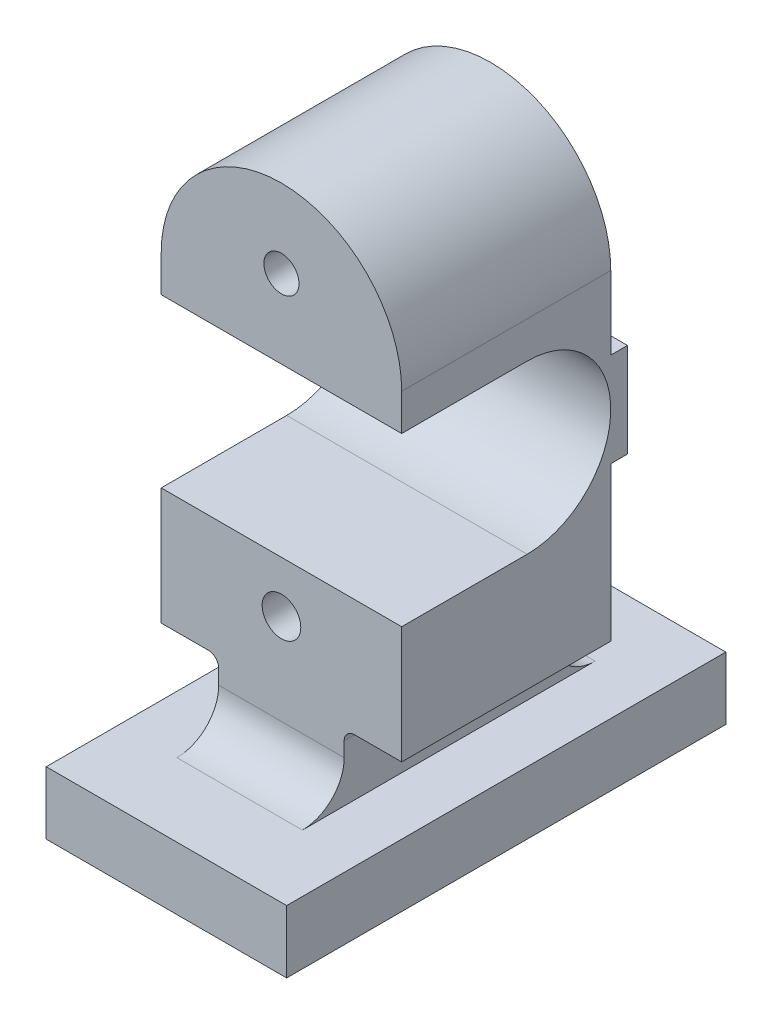
ISO-10303-21;
HEADER;
FILE_DESCRIPTION(('STEP AP214'),'2;1');
FILE_NAME('part.step','',(''),(''),'','','');
FILE_SCHEMA(('AUTOMOTIVE_DESIGN { 1 0 10303 214 1 1 1 1 }'));
ENDSEC;
DATA;
#1=APPLICATION_CONTEXT('core data for automotive mechanical design processes');
#2=APPLICATION_PROTOCOL_DEFINITION('international standard','automotive_design',2000,#1);
#3=PRODUCT_CONTEXT('',#1,'mechanical');
#4=PRODUCT('Part','Part','',(#3));
#5=PRODUCT_RELATED_PRODUCT_CATEGORY('part','',(#4));
#6=PRODUCT_DEFINITION_FORMATION('','',#4);
#7=PRODUCT_DEFINITION_CONTEXT('part definition',#1,'design');
#8=PRODUCT_DEFINITION('design','',#6,#7);
#9=PRODUCT_DEFINITION_SHAPE('','',#8);
#10=(LENGTH_UNIT() NAMED_UNIT(*) SI_UNIT(.MILLI.,.METRE.));
#11=(NAMED_UNIT(*) PLANE_ANGLE_UNIT() SI_UNIT($,.RADIAN.));
#12=(NAMED_UNIT(*) SI_UNIT($,.STERADIAN.) SOLID_ANGLE_UNIT());
#13=UNCERTAINTY_MEASURE_WITH_UNIT(LENGTH_MEASURE(1.E-05),#10,'distance_accuracy_value','');
#14=(GEOMETRIC_REPRESENTATION_CONTEXT(3) GLOBAL_UNCERTAINTY_ASSIGNED_CONTEXT((#13)) GLOBAL_UNIT_ASSIGNED_CONTEXT((#10,
#11,#12)) REPRESENTATION_CONTEXT('',''));
#15=CARTESIAN_POINT('',(0.,0.,0.));
#16=DIRECTION('',(0.,0.,1.));
#17=DIRECTION('',(1.,0.,0.));
#18=AXIS2_PLACEMENT_3D('',#15,#16,#17);
#19=CARTESIAN_POINT('',(35.0000000000001,42.,50.));
#20=DIRECTION('',(0.,0.,-1.));
#21=DIRECTION('',(-1.,0.,0.));
#22=AXIS2_PLACEMENT_3D('',#19,#20,#21);
#23=PLANE('',#22);
#24=CARTESIAN_POINT('',(0.,78.5,50.));
#25=DIRECTION('',(0.,0.,1.));
#26=DIRECTION('',(1.,0.,0.));
#27=AXIS2_PLACEMENT_3D('',#24,#25,#26);
#28=CIRCLE('',#27,9.24443485272175);
#29=CARTESIAN_POINT('',(9.24443485272181,78.5,50.));
#30=VERTEX_POINT('',#29);
#31=EDGE_CURVE('E348',#30,#30,#28,.T.);
#32=ORIENTED_EDGE('',*,*,#31,.F.);
#33=EDGE_LOOP('',(#32));
#34=FACE_BOUND('',#33,.T.);
#35=DIRECTION('',(0.,-1.,0.));
#36=VECTOR('',#35,1.);
#37=CARTESIAN_POINT('',(-29.9999999999999,42.,50.));
#38=LINE('',#37,#36);
#39=CARTESIAN_POINT('',(-29.9999999999999,42.,50.));
#40=VERTEX_POINT('',#39);
#41=CARTESIAN_POINT('',(-29.9999999999999,35.,50.));
#42=VERTEX_POINT('',#41);
#43=EDGE_CURVE('E361',#40,#42,#38,.T.);
#44=ORIENTED_EDGE('',*,*,#43,.T.);
#45=DIRECTION('',(1.,0.,0.));
#46=VECTOR('',#45,1.);
#47=CARTESIAN_POINT('',(35.0000000000001,35.,50.));
#48=LINE('',#47,#46);
#49=CARTESIAN_POINT('',(30.0000000000001,35.,50.));
#50=VERTEX_POINT('',#49);
#51=EDGE_CURVE('E393',#42,#50,#48,.T.);
#52=ORIENTED_EDGE('',*,*,#51,.T.);
#53=DIRECTION('',(0.,1.,0.));
#54=VECTOR('',#53,1.);
#55=CARTESIAN_POINT('',(30.0000000000001,42.,50.));
#56=LINE('',#55,#54);
#57=CARTESIAN_POINT('',(30.0000000000001,42.,50.));
#58=VERTEX_POINT('',#57);
#59=EDGE_CURVE('E363',#50,#58,#56,.T.);
#60=ORIENTED_EDGE('',*,*,#59,.T.);
#61=CARTESIAN_POINT('',(35.0000000000001,42.,50.));
#62=DIRECTION('',(0.,0.,-1.));
#63=DIRECTION('',(-1.,0.,0.));
#64=AXIS2_PLACEMENT_3D('',#61,#62,#63);
#65=CIRCLE('',#64,5.);
#66=CARTESIAN_POINT('',(35.0000000000001,47.,50.));
#67=VERTEX_POINT('',#66);
#68=EDGE_CURVE('E360',#58,#67,#65,.T.);
#69=ORIENTED_EDGE('',*,*,#68,.T.);
#70=DIRECTION('',(1.,0.,0.));
#71=VECTOR('',#70,1.);
#72=CARTESIAN_POINT('',(57.5,47.,50.));
#73=LINE('',#72,#71);
#74=CARTESIAN_POINT('',(57.5,47.,50.));
#75=VERTEX_POINT('',#74);
#76=EDGE_CURVE('E358',#67,#75,#73,.T.);
#77=ORIENTED_EDGE('',*,*,#76,.T.);
#78=DIRECTION('',(0.,1.,0.));
#79=VECTOR('',#78,1.);
#80=CARTESIAN_POINT('',(57.5,47.,50.));
#81=LINE('',#80,#79);
#82=CARTESIAN_POINT('',(57.5,103.,50.));
#83=VERTEX_POINT('',#82);
#84=EDGE_CURVE('E356',#75,#83,#81,.T.);
#85=ORIENTED_EDGE('',*,*,#84,.T.);
#86=DIRECTION('',(1.,0.,0.));
#87=VECTOR('',#86,1.);
#88=CARTESIAN_POINT('',(-75.,103.,50.));
#89=LINE('',#88,#87);
#90=CARTESIAN_POINT('',(-57.5,103.,50.));
#91=VERTEX_POINT('',#90);
#92=EDGE_CURVE('E373',#91,#83,#89,.T.);
#93=ORIENTED_EDGE('',*,*,#92,.F.);
#94=DIRECTION('',(0.,-1.,0.));
#95=VECTOR('',#94,1.);
#96=CARTESIAN_POINT('',(-57.5,47.,50.));
#97=LINE('',#96,#95);
#98=CARTESIAN_POINT('',(-57.5,47.,50.));
#99=VERTEX_POINT('',#98);
#100=EDGE_CURVE('E282',#91,#99,#97,.T.);
#101=ORIENTED_EDGE('',*,*,#100,.T.);
#102=DIRECTION('',(1.,0.,0.));
#103=VECTOR('',#102,1.);
#104=CARTESIAN_POINT('',(-34.9999999999999,47.,50.));
#105=LINE('',#104,#103);
#106=CARTESIAN_POINT('',(-34.9999999999999,47.,50.));
#107=VERTEX_POINT('',#106);
#108=EDGE_CURVE('E370',#99,#107,#105,.T.);
#109=ORIENTED_EDGE('',*,*,#108,.T.);
#110=CARTESIAN_POINT('',(-34.9999999999999,42.,50.));
#111=DIRECTION('',(0.,0.,-1.));
#112=DIRECTION('',(1.,0.,0.));
#113=AXIS2_PLACEMENT_3D('',#110,#111,#112);
#114=CIRCLE('',#113,5.);
#115=EDGE_CURVE('E362',#107,#40,#114,.T.);
#116=ORIENTED_EDGE('',*,*,#115,.T.);
#117=EDGE_LOOP('',(#44,#52,#60,#69,#77,#85,#93,#101,#109,#116));
#118=FACE_BOUND('',#117,.T.);
#119=ADVANCED_FACE('F41',(#34,#118),#23,.F.);
#120=CARTESIAN_POINT('',(35.0000000000001,42.,-50.));
#121=DIRECTION('',(0.,0.,-1.));
#122=DIRECTION('',(-1.,0.,0.));
#123=AXIS2_PLACEMENT_3D('',#120,#121,#122);
#124=PLANE('',#123);
#125=DIRECTION('',(0.,1.,0.));
#126=VECTOR('',#125,1.);
#127=CARTESIAN_POINT('',(30.0000000000001,42.,-50.));
#128=LINE('',#127,#126);
#129=CARTESIAN_POINT('',(30.0000000000001,35.,-50.));
#130=VERTEX_POINT('',#129);
#131=CARTESIAN_POINT('',(30.0000000000001,42.,-50.));
#132=VERTEX_POINT('',#131);
#133=EDGE_CURVE('E333',#130,#132,#128,.T.);
#134=ORIENTED_EDGE('',*,*,#133,.F.);
#135=DIRECTION('',(1.,0.,0.));
#136=VECTOR('',#135,1.);
#137=CARTESIAN_POINT('',(-29.9999999999999,35.,-50.));
#138=LINE('',#137,#136);
#139=CARTESIAN_POINT('',(-29.9999999999999,35.,-50.));
#140=VERTEX_POINT('',#139);
#141=EDGE_CURVE('E391',#130,#140,#138,.F.);
#142=ORIENTED_EDGE('',*,*,#141,.T.);
#143=DIRECTION('',(0.,-1.,0.));
#144=VECTOR('',#143,1.);
#145=CARTESIAN_POINT('',(-29.9999999999999,42.,-50.));
#146=LINE('',#145,#144);
#147=CARTESIAN_POINT('',(-29.9999999999999,42.,-50.));
#148=VERTEX_POINT('',#147);
#149=EDGE_CURVE('E327',#148,#140,#146,.T.);
#150=ORIENTED_EDGE('',*,*,#149,.F.);
#151=CARTESIAN_POINT('',(-34.9999999999999,42.,-50.));
#152=DIRECTION('',(0.,0.,-1.));
#153=DIRECTION('',(1.,0.,0.));
#154=AXIS2_PLACEMENT_3D('',#151,#152,#153);
#155=CIRCLE('',#154,5.);
#156=CARTESIAN_POINT('',(-34.9999999999999,47.,-50.));
#157=VERTEX_POINT('',#156);
#158=EDGE_CURVE('E321',#157,#148,#155,.T.);
#159=ORIENTED_EDGE('',*,*,#158,.F.);
#160=DIRECTION('',(1.,0.,0.));
#161=VECTOR('',#160,1.);
#162=CARTESIAN_POINT('',(-34.9999999999999,47.,-50.));
#163=LINE('',#162,#161);
#164=CARTESIAN_POINT('',(-57.5,47.,-50.));
#165=VERTEX_POINT('',#164);
#166=EDGE_CURVE('E323',#165,#157,#163,.T.);
#167=ORIENTED_EDGE('',*,*,#166,.F.);
#168=DIRECTION('',(0.,-1.,0.));
#169=VECTOR('',#168,1.);
#170=CARTESIAN_POINT('',(-57.5,47.,-50.));
#171=LINE('',#170,#169);
#172=CARTESIAN_POINT('',(-57.5,120.5,-50.));
#173=VERTEX_POINT('',#172);
#174=EDGE_CURVE('E211',#173,#165,#171,.T.);
#175=ORIENTED_EDGE('',*,*,#174,.F.);
#176=DIRECTION('',(-1.,0.,0.));
#177=VECTOR('',#176,1.);
#178=CARTESIAN_POINT('',(57.5,120.5,-50.));
#179=LINE('',#178,#177);
#180=CARTESIAN_POINT('',(57.5,120.5,-50.));
#181=VERTEX_POINT('',#180);
#182=EDGE_CURVE('E273',#181,#173,#179,.T.);
#183=ORIENTED_EDGE('',*,*,#182,.F.);
#184=DIRECTION('',(0.,1.,0.));
#185=VECTOR('',#184,1.);
#186=CARTESIAN_POINT('',(57.5,47.,-50.));
#187=LINE('',#186,#185);
#188=CARTESIAN_POINT('',(57.5,47.,-50.));
#189=VERTEX_POINT('',#188);
#190=EDGE_CURVE('E343',#189,#181,#187,.T.);
#191=ORIENTED_EDGE('',*,*,#190,.F.);
#192=DIRECTION('',(1.,0.,0.));
#193=VECTOR('',#192,1.);
#194=CARTESIAN_POINT('',(57.5,47.,-50.));
#195=LINE('',#194,#193);
#196=CARTESIAN_POINT('',(35.0000000000001,47.,-50.));
#197=VERTEX_POINT('',#196);
#198=EDGE_CURVE('E342',#197,#189,#195,.T.);
#199=ORIENTED_EDGE('',*,*,#198,.F.);
#200=CARTESIAN_POINT('',(35.0000000000001,42.,-50.));
#201=DIRECTION('',(0.,0.,-1.));
#202=DIRECTION('',(-1.,0.,0.));
#203=AXIS2_PLACEMENT_3D('',#200,#201,#202);
#204=CIRCLE('',#203,5.);
#205=EDGE_CURVE('E340',#132,#197,#204,.T.);
#206=ORIENTED_EDGE('',*,*,#205,.F.);
#207=EDGE_LOOP('',(#134,#142,#150,#159,#167,#175,#183,#191,#199,#206));
#208=FACE_BOUND('',#207,.T.);
#209=CARTESIAN_POINT('',(0.,78.5,-50.));
#210=DIRECTION('',(0.,0.,1.));
#211=DIRECTION('',(1.,0.,0.));
#212=AXIS2_PLACEMENT_3D('',#209,#210,#211);
#213=CIRCLE('',#212,9.24443485272175);
#214=CARTESIAN_POINT('',(9.24443485272181,78.5,-50.));
#215=VERTEX_POINT('',#214);
#216=EDGE_CURVE('E318',#215,#215,#213,.T.);
#217=ORIENTED_EDGE('',*,*,#216,.T.);
#218=EDGE_LOOP('',(#217));
#219=FACE_BOUND('',#218,.T.);
#220=ADVANCED_FACE('F412',(#208,#219),#124,.T.);
#221=CARTESIAN_POINT('',(0.,15.,0.));
#222=DIRECTION('',(0.,1.,0.));
#223=DIRECTION('',(0.,0.,1.));
#224=AXIS2_PLACEMENT_3D('',#221,#222,#223);
#225=PLANE('',#224);
#226=DIRECTION('',(0.,0.,-1.));
#227=VECTOR('',#226,1.);
#228=CARTESIAN_POINT('',(57.5,15.,-105.));
#229=LINE('',#228,#227);
#230=CARTESIAN_POINT('',(57.5,15.,105.));
#231=VERTEX_POINT('',#230);
#232=CARTESIAN_POINT('',(57.5,15.,-105.));
#233=VERTEX_POINT('',#232);
#234=EDGE_CURVE('E320',#231,#233,#229,.T.);
#235=ORIENTED_EDGE('',*,*,#234,.T.);
#236=DIRECTION('',(-1.,0.,0.));
#237=VECTOR('',#236,1.);
#238=CARTESIAN_POINT('',(-57.5,15.,-105.));
#239=LINE('',#238,#237);
#240=CARTESIAN_POINT('',(-57.5,15.,-105.));
#241=VERTEX_POINT('',#240);
#242=EDGE_CURVE('E314',#233,#241,#239,.T.);
#243=ORIENTED_EDGE('',*,*,#242,.T.);
#244=DIRECTION('',(0.,0.,1.));
#245=VECTOR('',#244,1.);
#246=CARTESIAN_POINT('',(-57.5,15.,-105.));
#247=LINE('',#246,#245);
#248=CARTESIAN_POINT('',(-57.5,15.,105.));
#249=VERTEX_POINT('',#248);
#250=EDGE_CURVE('E312',#241,#249,#247,.T.);
#251=ORIENTED_EDGE('',*,*,#250,.T.);
#252=DIRECTION('',(1.,0.,0.));
#253=VECTOR('',#252,1.);
#254=CARTESIAN_POINT('',(-57.5,15.,105.));
#255=LINE('',#254,#253);
#256=EDGE_CURVE('E311',#249,#231,#255,.T.);
#257=ORIENTED_EDGE('',*,*,#256,.T.);
#258=EDGE_LOOP('',(#235,#243,#251,#257));
#259=FACE_BOUND('',#258,.T.);
#260=DIRECTION('',(1.,0.,0.));
#261=VECTOR('',#260,1.);
#262=CARTESIAN_POINT('',(30.0000000000001,15.,-70.));
#263=LINE('',#262,#261);
#264=CARTESIAN_POINT('',(-29.9999999999999,15.,-70.));
#265=VERTEX_POINT('',#264);
#266=CARTESIAN_POINT('',(30.0000000000001,15.,-70.));
#267=VERTEX_POINT('',#266);
#268=EDGE_CURVE('E389',#265,#267,#263,.T.);
#269=ORIENTED_EDGE('',*,*,#268,.T.);
#270=DIRECTION('',(0.,0.,-1.));
#271=VECTOR('',#270,1.);
#272=CARTESIAN_POINT('',(30.0000000000001,15.,50.));
#273=LINE('',#272,#271);
#274=CARTESIAN_POINT('',(30.0000000000001,15.,70.));
#275=VERTEX_POINT('',#274);
#276=EDGE_CURVE('E331',#275,#267,#273,.T.);
#277=ORIENTED_EDGE('',*,*,#276,.F.);
#278=DIRECTION('',(1.,0.,0.));
#279=VECTOR('',#278,1.);
#280=CARTESIAN_POINT('',(0.,15.,70.));
#281=LINE('',#280,#279);
#282=CARTESIAN_POINT('',(-29.9999999999999,15.,70.));
#283=VERTEX_POINT('',#282);
#284=EDGE_CURVE('E377',#275,#283,#281,.F.);
#285=ORIENTED_EDGE('',*,*,#284,.T.);
#286=DIRECTION('',(0.,0.,-1.));
#287=VECTOR('',#286,1.);
#288=CARTESIAN_POINT('',(-29.9999999999999,15.,50.));
#289=LINE('',#288,#287);
#290=EDGE_CURVE('E309',#283,#265,#289,.T.);
#291=ORIENTED_EDGE('',*,*,#290,.T.);
#292=EDGE_LOOP('',(#269,#277,#285,#291));
#293=FACE_BOUND('',#292,.T.);
#294=ADVANCED_FACE('F403',(#259,#293),#225,.T.);
#295=CARTESIAN_POINT('',(57.5,15.,-105.));
#296=DIRECTION('',(-1.,0.,0.));
#297=DIRECTION('',(0.,0.,1.));
#298=AXIS2_PLACEMENT_3D('',#295,#296,#297);
#299=PLANE('',#298);
#300=DIRECTION('',(0.,0.,-1.));
#301=VECTOR('',#300,1.);
#302=CARTESIAN_POINT('',(57.5,-15.,-105.));
#303=LINE('',#302,#301);
#304=CARTESIAN_POINT('',(57.5,-15.,105.));
#305=VERTEX_POINT('',#304);
#306=CARTESIAN_POINT('',(57.5,-15.,-105.));
#307=VERTEX_POINT('',#306);
#308=EDGE_CURVE('E302',#305,#307,#303,.T.);
#309=ORIENTED_EDGE('',*,*,#308,.T.);
#310=DIRECTION('',(0.,-1.,0.));
#311=VECTOR('',#310,1.);
#312=CARTESIAN_POINT('',(57.5,15.,-105.));
#313=LINE('',#312,#311);
#314=EDGE_CURVE('E289',#233,#307,#313,.T.);
#315=ORIENTED_EDGE('',*,*,#314,.F.);
#316=ORIENTED_EDGE('',*,*,#234,.F.);
#317=DIRECTION('',(0.,-1.,0.));
#318=VECTOR('',#317,1.);
#319=CARTESIAN_POINT('',(57.5,15.,105.));
#320=LINE('',#319,#318);
#321=EDGE_CURVE('E301',#231,#305,#320,.T.);
#322=ORIENTED_EDGE('',*,*,#321,.T.);
#323=EDGE_LOOP('',(#309,#315,#316,#322));
#324=FACE_BOUND('',#323,.T.);
#325=ADVANCED_FACE('F511',(#324),#299,.F.);
#326=CARTESIAN_POINT('',(-57.5,15.,-105.));
#327=DIRECTION('',(0.,0.,1.));
#328=DIRECTION('',(1.,0.,0.));
#329=AXIS2_PLACEMENT_3D('',#326,#327,#328);
#330=PLANE('',#329);
#331=DIRECTION('',(-1.,0.,0.));
#332=VECTOR('',#331,1.);
#333=CARTESIAN_POINT('',(-57.5,-15.,-105.));
#334=LINE('',#333,#332);
#335=CARTESIAN_POINT('',(-57.5,-15.,-105.));
#336=VERTEX_POINT('',#335);
#337=EDGE_CURVE('E291',#307,#336,#334,.T.);
#338=ORIENTED_EDGE('',*,*,#337,.T.);
#339=DIRECTION('',(0.,-1.,0.));
#340=VECTOR('',#339,1.);
#341=CARTESIAN_POINT('',(-57.5,15.,-105.));
#342=LINE('',#341,#340);
#343=EDGE_CURVE('E295',#241,#336,#342,.T.);
#344=ORIENTED_EDGE('',*,*,#343,.F.);
#345=ORIENTED_EDGE('',*,*,#242,.F.);
#346=ORIENTED_EDGE('',*,*,#314,.T.);
#347=EDGE_LOOP('',(#338,#344,#345,#346));
#348=FACE_BOUND('',#347,.T.);
#349=ADVANCED_FACE('F520',(#348),#330,.F.);
#350=CARTESIAN_POINT('',(-57.5,15.,-105.));
#351=DIRECTION('',(1.,0.,0.));
#352=DIRECTION('',(0.,0.,-1.));
#353=AXIS2_PLACEMENT_3D('',#350,#351,#352);
#354=PLANE('',#353);
#355=DIRECTION('',(0.,0.,1.));
#356=VECTOR('',#355,1.);
#357=CARTESIAN_POINT('',(-57.5,-15.,-105.));
#358=LINE('',#357,#356);
#359=CARTESIAN_POINT('',(-57.5,-15.,105.));
#360=VERTEX_POINT('',#359);
#361=EDGE_CURVE('E292',#336,#360,#358,.T.);
#362=ORIENTED_EDGE('',*,*,#361,.T.);
#363=DIRECTION('',(0.,-1.,0.));
#364=VECTOR('',#363,1.);
#365=CARTESIAN_POINT('',(-57.5,15.,105.));
#366=LINE('',#365,#364);
#367=EDGE_CURVE('E296',#249,#360,#366,.T.);
#368=ORIENTED_EDGE('',*,*,#367,.F.);
#369=ORIENTED_EDGE('',*,*,#250,.F.);
#370=ORIENTED_EDGE('',*,*,#343,.T.);
#371=EDGE_LOOP('',(#362,#368,#369,#370));
#372=FACE_BOUND('',#371,.T.);
#373=ADVANCED_FACE('F521',(#372),#354,.F.);
#374=CARTESIAN_POINT('',(-57.5,15.,105.));
#375=DIRECTION('',(0.,0.,-1.));
#376=DIRECTION('',(-1.,0.,0.));
#377=AXIS2_PLACEMENT_3D('',#374,#375,#376);
#378=PLANE('',#377);
#379=DIRECTION('',(1.,0.,0.));
#380=VECTOR('',#379,1.);
#381=CARTESIAN_POINT('',(-57.5,-15.,105.));
#382=LINE('',#381,#380);
#383=EDGE_CURVE('E300',#360,#305,#382,.T.);
#384=ORIENTED_EDGE('',*,*,#383,.T.);
#385=ORIENTED_EDGE('',*,*,#321,.F.);
#386=ORIENTED_EDGE('',*,*,#256,.F.);
#387=ORIENTED_EDGE('',*,*,#367,.T.);
#388=EDGE_LOOP('',(#384,#385,#386,#387));
#389=FACE_BOUND('',#388,.T.);
#390=ADVANCED_FACE('F524',(#389),#378,.F.);
#391=CARTESIAN_POINT('',(0.,-15.,0.));
#392=DIRECTION('',(0.,1.,0.));
#393=DIRECTION('',(0.,0.,1.));
#394=AXIS2_PLACEMENT_3D('',#391,#392,#393);
#395=PLANE('',#394);
#396=ORIENTED_EDGE('',*,*,#308,.F.);
#397=ORIENTED_EDGE('',*,*,#383,.F.);
#398=ORIENTED_EDGE('',*,*,#361,.F.);
#399=ORIENTED_EDGE('',*,*,#337,.F.);
#400=EDGE_LOOP('',(#396,#397,#398,#399));
#401=FACE_BOUND('',#400,.T.);
#402=ADVANCED_FACE('F529',(#401),#395,.F.);
#403=CARTESIAN_POINT('',(-57.5,47.,50.));
#404=DIRECTION('',(1.,0.,0.));
#405=DIRECTION('',(0.,1.,0.));
#406=AXIS2_PLACEMENT_3D('',#403,#404,#405);
#407=PLANE('',#406);
#408=DIRECTION('',(0.,0.,-1.));
#409=VECTOR('',#408,1.);
#410=CARTESIAN_POINT('',(-57.5,103.,50.));
#411=LINE('',#410,#409);
#412=CARTESIAN_POINT('',(-57.5,103.,-9.99999999999999));
#413=VERTEX_POINT('',#412);
#414=EDGE_CURVE('E209',#91,#413,#411,.T.);
#415=ORIENTED_EDGE('',*,*,#414,.T.);
#416=CARTESIAN_POINT('',(-57.5,143.,-10.));
#417=DIRECTION('',(1.,0.,0.));
#418=DIRECTION('',(0.,1.,0.));
#419=AXIS2_PLACEMENT_3D('',#416,#417,#418);
#420=CIRCLE('',#419,40.);
#421=CARTESIAN_POINT('',(-57.5,183.,-9.99999999999999));
#422=VERTEX_POINT('',#421);
#423=EDGE_CURVE('E205',#413,#422,#420,.T.);
#424=ORIENTED_EDGE('',*,*,#423,.T.);
#425=DIRECTION('',(0.,0.,1.));
#426=VECTOR('',#425,1.);
#427=CARTESIAN_POINT('',(-57.5,183.,50.));
#428=LINE('',#427,#426);
#429=CARTESIAN_POINT('',(-57.5,183.,50.));
#430=VERTEX_POINT('',#429);
#431=EDGE_CURVE('E207',#422,#430,#428,.T.);
#432=ORIENTED_EDGE('',*,*,#431,.T.);
#433=DIRECTION('',(0.,-1.,0.));
#434=VECTOR('',#433,1.);
#435=CARTESIAN_POINT('',(-57.5,47.,50.));
#436=LINE('',#435,#434);
#437=CARTESIAN_POINT('',(-57.5,200.5,50.));
#438=VERTEX_POINT('',#437);
#439=EDGE_CURVE('E240',#438,#430,#436,.T.);
#440=ORIENTED_EDGE('',*,*,#439,.F.);
#441=DIRECTION('',(0.,0.,-1.));
#442=VECTOR('',#441,1.);
#443=CARTESIAN_POINT('',(-57.5,200.5,50.));
#444=LINE('',#443,#442);
#445=CARTESIAN_POINT('',(-57.5,200.5,-50.));
#446=VERTEX_POINT('',#445);
#447=EDGE_CURVE('E245',#438,#446,#444,.T.);
#448=ORIENTED_EDGE('',*,*,#447,.T.);
#449=DIRECTION('',(0.,-1.,0.));
#450=VECTOR('',#449,1.);
#451=CARTESIAN_POINT('',(-57.5,47.,-50.));
#452=LINE('',#451,#450);
#453=CARTESIAN_POINT('',(-57.5,165.5,-50.));
#454=VERTEX_POINT('',#453);
#455=EDGE_CURVE('E234',#446,#454,#452,.T.);
#456=ORIENTED_EDGE('',*,*,#455,.T.);
#457=DIRECTION('',(0.,0.,1.));
#458=VECTOR('',#457,1.);
#459=CARTESIAN_POINT('',(-57.5,165.5,-50.));
#460=LINE('',#459,#458);
#461=CARTESIAN_POINT('',(-57.5,165.5,-58.));
#462=VERTEX_POINT('',#461);
#463=EDGE_CURVE('E266',#462,#454,#460,.T.);
#464=ORIENTED_EDGE('',*,*,#463,.F.);
#465=DIRECTION('',(0.,1.,0.));
#466=VECTOR('',#465,1.);
#467=CARTESIAN_POINT('',(-57.5,120.5,-58.));
#468=LINE('',#467,#466);
#469=CARTESIAN_POINT('',(-57.5,120.5,-58.));
#470=VERTEX_POINT('',#469);
#471=EDGE_CURVE('E259',#470,#462,#468,.T.);
#472=ORIENTED_EDGE('',*,*,#471,.F.);
#473=DIRECTION('',(0.,0.,-1.));
#474=VECTOR('',#473,1.);
#475=CARTESIAN_POINT('',(-57.5,120.5,-50.));
#476=LINE('',#475,#474);
#477=EDGE_CURVE('E263',#173,#470,#476,.T.);
#478=ORIENTED_EDGE('',*,*,#477,.F.);
#479=ORIENTED_EDGE('',*,*,#174,.T.);
#480=DIRECTION('',(0.,0.,-1.));
#481=VECTOR('',#480,1.);
#482=CARTESIAN_POINT('',(-57.5,47.,50.));
#483=LINE('',#482,#481);
#484=EDGE_CURVE('E322',#99,#165,#483,.T.);
#485=ORIENTED_EDGE('',*,*,#484,.F.);
#486=ORIENTED_EDGE('',*,*,#100,.F.);
#487=EDGE_LOOP('',(#415,#424,#432,#440,#448,#456,#464,#472,#478,#479,#485,#486));
#488=FACE_BOUND('',#487,.T.);
#489=ADVANCED_FACE('F204',(#488),#407,.F.);
#490=CARTESIAN_POINT('',(-34.9999999999999,47.,50.));
#491=DIRECTION('',(0.,1.,0.));
#492=DIRECTION('',(-1.,0.,0.));
#493=AXIS2_PLACEMENT_3D('',#490,#491,#492);
#494=PLANE('',#493);
#495=ORIENTED_EDGE('',*,*,#166,.T.);
#496=DIRECTION('',(0.,0.,-1.));
#497=VECTOR('',#496,1.);
#498=CARTESIAN_POINT('',(-34.9999999999999,47.,50.));
#499=LINE('',#498,#497);
#500=EDGE_CURVE('E326',#107,#157,#499,.T.);
#501=ORIENTED_EDGE('',*,*,#500,.F.);
#502=ORIENTED_EDGE('',*,*,#108,.F.);
#503=ORIENTED_EDGE('',*,*,#484,.T.);
#504=EDGE_LOOP('',(#495,#501,#502,#503));
#505=FACE_BOUND('',#504,.T.);
#506=ADVANCED_FACE('F439',(#505),#494,.F.);
#507=CARTESIAN_POINT('',(-34.9999999999999,42.,50.));
#508=DIRECTION('',(0.,0.,-1.));
#509=DIRECTION('',(-1.,0.,0.));
#510=AXIS2_PLACEMENT_3D('',#507,#508,#509);
#511=CYLINDRICAL_SURFACE('',#510,5.);
#512=ORIENTED_EDGE('',*,*,#158,.T.);
#513=DIRECTION('',(0.,0.,-1.));
#514=VECTOR('',#513,1.);
#515=CARTESIAN_POINT('',(-29.9999999999999,42.,50.));
#516=LINE('',#515,#514);
#517=EDGE_CURVE('E329',#40,#148,#516,.T.);
#518=ORIENTED_EDGE('',*,*,#517,.F.);
#519=ORIENTED_EDGE('',*,*,#115,.F.);
#520=ORIENTED_EDGE('',*,*,#500,.T.);
#521=EDGE_LOOP('',(#512,#518,#519,#520));
#522=FACE_BOUND('',#521,.T.);
#523=ADVANCED_FACE('F436',(#522),#511,.F.);
#524=CARTESIAN_POINT('',(-29.9999999999999,42.,50.));
#525=DIRECTION('',(1.,0.,0.));
#526=DIRECTION('',(0.,1.,0.));
#527=AXIS2_PLACEMENT_3D('',#524,#525,#526);
#528=PLANE('',#527);
#529=ORIENTED_EDGE('',*,*,#149,.T.);
#530=CARTESIAN_POINT('',(-29.9999999999999,35.,-70.));
#531=DIRECTION('',(1.,0.,0.));
#532=DIRECTION('',(0.,1.,0.));
#533=AXIS2_PLACEMENT_3D('',#530,#531,#532);
#534=CIRCLE('',#533,20.);
#535=EDGE_CURVE('E400',#140,#265,#534,.T.);
#536=ORIENTED_EDGE('',*,*,#535,.T.);
#537=ORIENTED_EDGE('',*,*,#290,.F.);
#538=CARTESIAN_POINT('',(-29.9999999999999,35.,70.));
#539=DIRECTION('',(1.,0.,0.));
#540=DIRECTION('',(0.,1.,0.));
#541=AXIS2_PLACEMENT_3D('',#538,#539,#540);
#542=CIRCLE('',#541,20.);
#543=EDGE_CURVE('E11',#283,#42,#542,.T.);
#544=ORIENTED_EDGE('',*,*,#543,.T.);
#545=ORIENTED_EDGE('',*,*,#43,.F.);
#546=ORIENTED_EDGE('',*,*,#517,.T.);
#547=EDGE_LOOP('',(#529,#536,#537,#544,#545,#546));
#548=FACE_BOUND('',#547,.T.);
#549=ADVANCED_FACE('F435',(#548),#528,.F.);
#550=CARTESIAN_POINT('',(30.0000000000001,42.,50.));
#551=DIRECTION('',(-1.,0.,0.));
#552=DIRECTION('',(0.,0.,1.));
#553=AXIS2_PLACEMENT_3D('',#550,#551,#552);
#554=PLANE('',#553);
#555=ORIENTED_EDGE('',*,*,#276,.T.);
#556=CARTESIAN_POINT('',(30.0000000000001,35.,-70.));
#557=DIRECTION('',(-1.,0.,0.));
#558=DIRECTION('',(0.,0.,1.));
#559=AXIS2_PLACEMENT_3D('',#556,#557,#558);
#560=CIRCLE('',#559,20.);
#561=EDGE_CURVE('E394',#267,#130,#560,.T.);
#562=ORIENTED_EDGE('',*,*,#561,.T.);
#563=ORIENTED_EDGE('',*,*,#133,.T.);
#564=DIRECTION('',(0.,0.,-1.));
#565=VECTOR('',#564,1.);
#566=CARTESIAN_POINT('',(30.0000000000001,42.,50.));
#567=LINE('',#566,#565);
#568=EDGE_CURVE('E336',#58,#132,#567,.T.);
#569=ORIENTED_EDGE('',*,*,#568,.F.);
#570=ORIENTED_EDGE('',*,*,#59,.F.);
#571=CARTESIAN_POINT('',(30.0000000000001,35.,70.));
#572=DIRECTION('',(-1.,0.,0.));
#573=DIRECTION('',(0.,0.,1.));
#574=AXIS2_PLACEMENT_3D('',#571,#572,#573);
#575=CIRCLE('',#574,20.);
#576=EDGE_CURVE('E47',#50,#275,#575,.T.);
#577=ORIENTED_EDGE('',*,*,#576,.T.);
#578=EDGE_LOOP('',(#555,#562,#563,#569,#570,#577));
#579=FACE_BOUND('',#578,.T.);
#580=ADVANCED_FACE('F402',(#579),#554,.F.);
#581=CARTESIAN_POINT('',(35.0000000000001,42.,50.));
#582=DIRECTION('',(0.,0.,-1.));
#583=DIRECTION('',(-1.,0.,0.));
#584=AXIS2_PLACEMENT_3D('',#581,#582,#583);
#585=CYLINDRICAL_SURFACE('',#584,5.);
#586=ORIENTED_EDGE('',*,*,#205,.T.);
#587=DIRECTION('',(0.,0.,-1.));
#588=VECTOR('',#587,1.);
#589=CARTESIAN_POINT('',(35.0000000000001,47.,50.));
#590=LINE('',#589,#588);
#591=EDGE_CURVE('E345',#67,#197,#590,.T.);
#592=ORIENTED_EDGE('',*,*,#591,.F.);
#593=ORIENTED_EDGE('',*,*,#68,.F.);
#594=ORIENTED_EDGE('',*,*,#568,.T.);
#595=EDGE_LOOP('',(#586,#592,#593,#594));
#596=FACE_BOUND('',#595,.T.);
#597=ADVANCED_FACE('F423',(#596),#585,.F.);
#598=CARTESIAN_POINT('',(57.5,47.,50.));
#599=DIRECTION('',(0.,1.,0.));
#600=DIRECTION('',(-1.,0.,0.));
#601=AXIS2_PLACEMENT_3D('',#598,#599,#600);
#602=PLANE('',#601);
#603=ORIENTED_EDGE('',*,*,#198,.T.);
#604=DIRECTION('',(0.,0.,-1.));
#605=VECTOR('',#604,1.);
#606=CARTESIAN_POINT('',(57.5,47.,50.));
#607=LINE('',#606,#605);
#608=EDGE_CURVE('E288',#75,#189,#607,.T.);
#609=ORIENTED_EDGE('',*,*,#608,.F.);
#610=ORIENTED_EDGE('',*,*,#76,.F.);
#611=ORIENTED_EDGE('',*,*,#591,.T.);
#612=EDGE_LOOP('',(#603,#609,#610,#611));
#613=FACE_BOUND('',#612,.T.);
#614=ADVANCED_FACE('F424',(#613),#602,.F.);
#615=CARTESIAN_POINT('',(57.5,47.,50.));
#616=DIRECTION('',(-1.,0.,0.));
#617=DIRECTION('',(0.,-1.,0.));
#618=AXIS2_PLACEMENT_3D('',#615,#616,#617);
#619=PLANE('',#618);
#620=ORIENTED_EDGE('',*,*,#190,.T.);
#621=DIRECTION('',(0.,0.,-1.));
#622=VECTOR('',#621,1.);
#623=CARTESIAN_POINT('',(57.5,120.5,-50.));
#624=LINE('',#623,#622);
#625=CARTESIAN_POINT('',(57.5,120.5,-58.));
#626=VERTEX_POINT('',#625);
#627=EDGE_CURVE('E264',#181,#626,#624,.T.);
#628=ORIENTED_EDGE('',*,*,#627,.T.);
#629=DIRECTION('',(0.,1.,0.));
#630=VECTOR('',#629,1.);
#631=CARTESIAN_POINT('',(57.5,120.5,-58.));
#632=LINE('',#631,#630);
#633=CARTESIAN_POINT('',(57.5,165.5,-58.));
#634=VERTEX_POINT('',#633);
#635=EDGE_CURVE('E256',#626,#634,#632,.T.);
#636=ORIENTED_EDGE('',*,*,#635,.T.);
#637=DIRECTION('',(0.,0.,1.));
#638=VECTOR('',#637,1.);
#639=CARTESIAN_POINT('',(57.5,165.5,-50.));
#640=LINE('',#639,#638);
#641=CARTESIAN_POINT('',(57.5,165.5,-50.));
#642=VERTEX_POINT('',#641);
#643=EDGE_CURVE('E265',#634,#642,#640,.T.);
#644=ORIENTED_EDGE('',*,*,#643,.T.);
#645=DIRECTION('',(0.,1.,0.));
#646=VECTOR('',#645,1.);
#647=CARTESIAN_POINT('',(57.5,47.,-50.));
#648=LINE('',#647,#646);
#649=CARTESIAN_POINT('',(57.5,200.5,-50.));
#650=VERTEX_POINT('',#649);
#651=EDGE_CURVE('E239',#642,#650,#648,.T.);
#652=ORIENTED_EDGE('',*,*,#651,.T.);
#653=DIRECTION('',(0.,0.,-1.));
#654=VECTOR('',#653,1.);
#655=CARTESIAN_POINT('',(57.5,200.5,50.));
#656=LINE('',#655,#654);
#657=CARTESIAN_POINT('',(57.5,200.5,50.));
#658=VERTEX_POINT('',#657);
#659=EDGE_CURVE('E247',#650,#658,#656,.F.);
#660=ORIENTED_EDGE('',*,*,#659,.T.);
#661=DIRECTION('',(0.,1.,0.));
#662=VECTOR('',#661,1.);
#663=CARTESIAN_POINT('',(57.5,47.,50.));
#664=LINE('',#663,#662);
#665=CARTESIAN_POINT('',(57.5,183.,50.));
#666=VERTEX_POINT('',#665);
#667=EDGE_CURVE('E237',#666,#658,#664,.T.);
#668=ORIENTED_EDGE('',*,*,#667,.F.);
#669=DIRECTION('',(0.,0.,-1.));
#670=VECTOR('',#669,1.);
#671=CARTESIAN_POINT('',(57.5,183.,50.));
#672=LINE('',#671,#670);
#673=CARTESIAN_POINT('',(57.5,183.,-9.99999999999999));
#674=VERTEX_POINT('',#673);
#675=EDGE_CURVE('E257',#666,#674,#672,.T.);
#676=ORIENTED_EDGE('',*,*,#675,.T.);
#677=CARTESIAN_POINT('',(57.5,143.,-10.));
#678=DIRECTION('',(-1.,0.,0.));
#679=DIRECTION('',(0.,-1.,0.));
#680=AXIS2_PLACEMENT_3D('',#677,#678,#679);
#681=CIRCLE('',#680,40.);
#682=CARTESIAN_POINT('',(57.5,103.,-9.99999999999999));
#683=VERTEX_POINT('',#682);
#684=EDGE_CURVE('E227',#674,#683,#681,.T.);
#685=ORIENTED_EDGE('',*,*,#684,.T.);
#686=DIRECTION('',(0.,0.,1.));
#687=VECTOR('',#686,1.);
#688=CARTESIAN_POINT('',(57.5,103.,50.));
#689=LINE('',#688,#687);
#690=EDGE_CURVE('E284',#683,#83,#689,.T.);
#691=ORIENTED_EDGE('',*,*,#690,.T.);
#692=ORIENTED_EDGE('',*,*,#84,.F.);
#693=ORIENTED_EDGE('',*,*,#608,.T.);
#694=EDGE_LOOP('',(#620,#628,#636,#644,#652,#660,#668,#676,#685,#691,#692,#693));
#695=FACE_BOUND('',#694,.T.);
#696=ADVANCED_FACE('F448',(#695),#619,.F.);
#697=CARTESIAN_POINT('',(0.,78.5,50.));
#698=DIRECTION('',(0.,0.,-1.));
#699=DIRECTION('',(-1.,0.,0.));
#700=AXIS2_PLACEMENT_3D('',#697,#698,#699);
#701=CYLINDRICAL_SURFACE('',#700,9.24443485272175);
#702=ORIENTED_EDGE('',*,*,#31,.T.);
#703=EDGE_LOOP('',(#702));
#704=FACE_BOUND('',#703,.T.);
#705=ORIENTED_EDGE('',*,*,#216,.F.);
#706=EDGE_LOOP('',(#705));
#707=FACE_BOUND('',#706,.T.);
#708=ADVANCED_FACE('F453',(#704,#707),#701,.F.);
#709=CARTESIAN_POINT('',(-75.,103.,50.));
#710=DIRECTION('',(0.,-1.,0.));
#711=DIRECTION('',(0.,0.,-1.));
#712=AXIS2_PLACEMENT_3D('',#709,#710,#711);
#713=PLANE('',#712);
#714=ORIENTED_EDGE('',*,*,#92,.T.);
#715=ORIENTED_EDGE('',*,*,#690,.F.);
#716=DIRECTION('',(1.,0.,0.));
#717=VECTOR('',#716,1.);
#718=CARTESIAN_POINT('',(-75.,103.,-9.99999999999999));
#719=LINE('',#718,#717);
#720=EDGE_CURVE('E376',#413,#683,#719,.T.);
#721=ORIENTED_EDGE('',*,*,#720,.F.);
#722=ORIENTED_EDGE('',*,*,#414,.F.);
#723=EDGE_LOOP('',(#714,#715,#721,#722));
#724=FACE_BOUND('',#723,.T.);
#725=ADVANCED_FACE('F454',(#724),#713,.F.);
#726=CARTESIAN_POINT('',(-75.,143.,-10.));
#727=DIRECTION('',(1.,0.,0.));
#728=DIRECTION('',(0.,0.,-1.));
#729=AXIS2_PLACEMENT_3D('',#726,#727,#728);
#730=CYLINDRICAL_SURFACE('',#729,40.);
#731=ORIENTED_EDGE('',*,*,#423,.F.);
#732=ORIENTED_EDGE('',*,*,#720,.T.);
#733=ORIENTED_EDGE('',*,*,#684,.F.);
#734=DIRECTION('',(1.,0.,0.));
#735=VECTOR('',#734,1.);
#736=CARTESIAN_POINT('',(-75.,183.,-9.99999999999999));
#737=LINE('',#736,#735);
#738=EDGE_CURVE('E217',#422,#674,#737,.T.);
#739=ORIENTED_EDGE('',*,*,#738,.F.);
#740=EDGE_LOOP('',(#731,#732,#733,#739));
#741=FACE_BOUND('',#740,.T.);
#742=ADVANCED_FACE('F221',(#741),#730,.F.);
#743=CARTESIAN_POINT('',(57.5,120.5,-58.));
#744=DIRECTION('',(0.,0.,1.));
#745=DIRECTION('',(1.,0.,0.));
#746=AXIS2_PLACEMENT_3D('',#743,#744,#745);
#747=PLANE('',#746);
#748=ORIENTED_EDGE('',*,*,#471,.T.);
#749=DIRECTION('',(-1.,0.,0.));
#750=VECTOR('',#749,1.);
#751=CARTESIAN_POINT('',(57.5,165.5,-58.));
#752=LINE('',#751,#750);
#753=EDGE_CURVE('E281',#634,#462,#752,.T.);
#754=ORIENTED_EDGE('',*,*,#753,.F.);
#755=ORIENTED_EDGE('',*,*,#635,.F.);
#756=DIRECTION('',(-1.,0.,0.));
#757=VECTOR('',#756,1.);
#758=CARTESIAN_POINT('',(57.5,120.5,-58.));
#759=LINE('',#758,#757);
#760=EDGE_CURVE('E270',#626,#470,#759,.T.);
#761=ORIENTED_EDGE('',*,*,#760,.T.);
#762=EDGE_LOOP('',(#748,#754,#755,#761));
#763=FACE_BOUND('',#762,.T.);
#764=ADVANCED_FACE('F465',(#763),#747,.F.);
#765=CARTESIAN_POINT('',(57.5,165.5,-50.));
#766=DIRECTION('',(0.,-1.,0.));
#767=DIRECTION('',(0.,0.,-1.));
#768=AXIS2_PLACEMENT_3D('',#765,#766,#767);
#769=PLANE('',#768);
#770=ORIENTED_EDGE('',*,*,#463,.T.);
#771=DIRECTION('',(-1.,0.,0.));
#772=VECTOR('',#771,1.);
#773=CARTESIAN_POINT('',(57.5,165.5,-50.));
#774=LINE('',#773,#772);
#775=EDGE_CURVE('E279',#642,#454,#774,.T.);
#776=ORIENTED_EDGE('',*,*,#775,.F.);
#777=ORIENTED_EDGE('',*,*,#643,.F.);
#778=ORIENTED_EDGE('',*,*,#753,.T.);
#779=EDGE_LOOP('',(#770,#776,#777,#778));
#780=FACE_BOUND('',#779,.T.);
#781=ADVANCED_FACE('F510',(#780),#769,.F.);
#782=CARTESIAN_POINT('',(57.5,120.5,-50.));
#783=DIRECTION('',(0.,1.,0.));
#784=DIRECTION('',(0.,0.,1.));
#785=AXIS2_PLACEMENT_3D('',#782,#783,#784);
#786=PLANE('',#785);
#787=ORIENTED_EDGE('',*,*,#477,.T.);
#788=ORIENTED_EDGE('',*,*,#760,.F.);
#789=ORIENTED_EDGE('',*,*,#627,.F.);
#790=ORIENTED_EDGE('',*,*,#182,.T.);
#791=EDGE_LOOP('',(#787,#788,#789,#790));
#792=FACE_BOUND('',#791,.T.);
#793=ADVANCED_FACE('F447',(#792),#786,.F.);
#794=CARTESIAN_POINT('',(0.,220.5,50.));
#795=DIRECTION('',(0.,0.,-1.));
#796=DIRECTION('',(-1.,0.,0.));
#797=AXIS2_PLACEMENT_3D('',#794,#795,#796);
#798=CYLINDRICAL_SURFACE('',#797,8.39406910894028);
#799=CARTESIAN_POINT('',(0.,220.5,50.));
#800=DIRECTION('',(0.,0.,1.));
#801=DIRECTION('',(1.,0.,0.));
#802=AXIS2_PLACEMENT_3D('',#799,#800,#801);
#803=CIRCLE('',#802,8.39406910894028);
#804=CARTESIAN_POINT('',(8.39406910894032,220.5,50.));
#805=VERTEX_POINT('',#804);
#806=EDGE_CURVE('E233',#805,#805,#803,.T.);
#807=ORIENTED_EDGE('',*,*,#806,.T.);
#808=EDGE_LOOP('',(#807));
#809=FACE_BOUND('',#808,.T.);
#810=CARTESIAN_POINT('',(0.,220.5,-50.));
#811=DIRECTION('',(0.,0.,1.));
#812=DIRECTION('',(1.,0.,0.));
#813=AXIS2_PLACEMENT_3D('',#810,#811,#812);
#814=CIRCLE('',#813,8.39406910894028);
#815=CARTESIAN_POINT('',(8.39406910894032,220.5,-50.));
#816=VERTEX_POINT('',#815);
#817=EDGE_CURVE('E223',#816,#816,#814,.T.);
#818=ORIENTED_EDGE('',*,*,#817,.F.);
#819=EDGE_LOOP('',(#818));
#820=FACE_BOUND('',#819,.T.);
#821=ADVANCED_FACE('F493',(#809,#820),#798,.F.);
#822=CARTESIAN_POINT('',(0.,200.5,50.));
#823=DIRECTION('',(0.,0.,-1.));
#824=DIRECTION('',(-1.,0.,0.));
#825=AXIS2_PLACEMENT_3D('',#822,#823,#824);
#826=CYLINDRICAL_SURFACE('',#825,57.5);
#827=ORIENTED_EDGE('',*,*,#447,.F.);
#828=CARTESIAN_POINT('',(0.,200.5,50.));
#829=DIRECTION('',(0.,0.,-1.));
#830=DIRECTION('',(-1.,0.,0.));
#831=AXIS2_PLACEMENT_3D('',#828,#829,#830);
#832=CIRCLE('',#831,57.5);
#833=EDGE_CURVE('E252',#658,#438,#832,.F.);
#834=ORIENTED_EDGE('',*,*,#833,.F.);
#835=ORIENTED_EDGE('',*,*,#659,.F.);
#836=CARTESIAN_POINT('',(0.,200.5,-50.));
#837=DIRECTION('',(0.,0.,-1.));
#838=DIRECTION('',(-1.,0.,0.));
#839=AXIS2_PLACEMENT_3D('',#836,#837,#838);
#840=CIRCLE('',#839,57.5);
#841=EDGE_CURVE('E254',#446,#650,#840,.T.);
#842=ORIENTED_EDGE('',*,*,#841,.F.);
#843=EDGE_LOOP('',(#827,#834,#835,#842));
#844=FACE_BOUND('',#843,.T.);
#845=ADVANCED_FACE('F491',(#844),#826,.T.);
#846=CARTESIAN_POINT('',(35.0000000000001,42.,-50.));
#847=DIRECTION('',(0.,0.,-1.));
#848=DIRECTION('',(-1.,0.,0.));
#849=AXIS2_PLACEMENT_3D('',#846,#847,#848);
#850=PLANE('',#849);
#851=ORIENTED_EDGE('',*,*,#651,.F.);
#852=ORIENTED_EDGE('',*,*,#775,.T.);
#853=ORIENTED_EDGE('',*,*,#455,.F.);
#854=ORIENTED_EDGE('',*,*,#841,.T.);
#855=EDGE_LOOP('',(#851,#852,#853,#854));
#856=FACE_BOUND('',#855,.T.);
#857=ORIENTED_EDGE('',*,*,#817,.T.);
#858=EDGE_LOOP('',(#857));
#859=FACE_BOUND('',#858,.T.);
#860=ADVANCED_FACE('F487',(#856,#859),#850,.T.);
#861=CARTESIAN_POINT('',(35.0000000000001,42.,50.));
#862=DIRECTION('',(0.,0.,-1.));
#863=DIRECTION('',(-1.,0.,0.));
#864=AXIS2_PLACEMENT_3D('',#861,#862,#863);
#865=PLANE('',#864);
#866=ORIENTED_EDGE('',*,*,#439,.T.);
#867=DIRECTION('',(1.,0.,0.));
#868=VECTOR('',#867,1.);
#869=CARTESIAN_POINT('',(-75.,183.,50.));
#870=LINE('',#869,#868);
#871=EDGE_CURVE('E225',#430,#666,#870,.T.);
#872=ORIENTED_EDGE('',*,*,#871,.T.);
#873=ORIENTED_EDGE('',*,*,#667,.T.);
#874=ORIENTED_EDGE('',*,*,#833,.T.);
#875=EDGE_LOOP('',(#866,#872,#873,#874));
#876=FACE_BOUND('',#875,.T.);
#877=ORIENTED_EDGE('',*,*,#806,.F.);
#878=EDGE_LOOP('',(#877));
#879=FACE_BOUND('',#878,.T.);
#880=ADVANCED_FACE('F485',(#876,#879),#865,.F.);
#881=CARTESIAN_POINT('',(-75.,183.,50.));
#882=DIRECTION('',(0.,1.,0.));
#883=DIRECTION('',(0.,0.,1.));
#884=AXIS2_PLACEMENT_3D('',#881,#882,#883);
#885=PLANE('',#884);
#886=ORIENTED_EDGE('',*,*,#738,.T.);
#887=ORIENTED_EDGE('',*,*,#675,.F.);
#888=ORIENTED_EDGE('',*,*,#871,.F.);
#889=ORIENTED_EDGE('',*,*,#431,.F.);
#890=EDGE_LOOP('',(#886,#887,#888,#889));
#891=FACE_BOUND('',#890,.T.);
#892=ADVANCED_FACE('F218',(#891),#885,.F.);
#893=CARTESIAN_POINT('',(0.,35.,-70.));
#894=DIRECTION('',(-1.,0.,0.));
#895=DIRECTION('',(0.,0.,1.));
#896=AXIS2_PLACEMENT_3D('',#893,#894,#895);
#897=CYLINDRICAL_SURFACE('',#896,20.);
#898=ORIENTED_EDGE('',*,*,#535,.F.);
#899=ORIENTED_EDGE('',*,*,#141,.F.);
#900=ORIENTED_EDGE('',*,*,#561,.F.);
#901=ORIENTED_EDGE('',*,*,#268,.F.);
#902=EDGE_LOOP('',(#898,#899,#900,#901));
#903=FACE_BOUND('',#902,.T.);
#904=ADVANCED_FACE('F406',(#903),#897,.F.);
#905=CARTESIAN_POINT('',(35.0000000000001,35.,70.));
#906=DIRECTION('',(1.,0.,0.));
#907=DIRECTION('',(0.,0.,-1.));
#908=AXIS2_PLACEMENT_3D('',#905,#906,#907);
#909=CYLINDRICAL_SURFACE('',#908,20.);
#910=ORIENTED_EDGE('',*,*,#543,.F.);
#911=ORIENTED_EDGE('',*,*,#284,.F.);
#912=ORIENTED_EDGE('',*,*,#576,.F.);
#913=ORIENTED_EDGE('',*,*,#51,.F.);
#914=EDGE_LOOP('',(#910,#911,#912,#913));
#915=FACE_BOUND('',#914,.T.);
#916=ADVANCED_FACE('F43',(#915),#909,.F.);
#917=CLOSED_SHELL('',(#119,#220,#294,#325,#349,#373,#390,#402,#489,#506,#523,#549,#580,#597,
#614,#696,#708,#725,#742,#764,#781,#793,#821,#845,#860,#880,#892,#904,#916));
#918=MANIFOLD_SOLID_BREP('B2',#917);
#919=ADVANCED_BREP_SHAPE_REPRESENTATION('',(#18,#918),#14);
#920=SHAPE_DEFINITION_REPRESENTATION(#9,#919);
ENDSEC;
END-ISO-10303-21;
